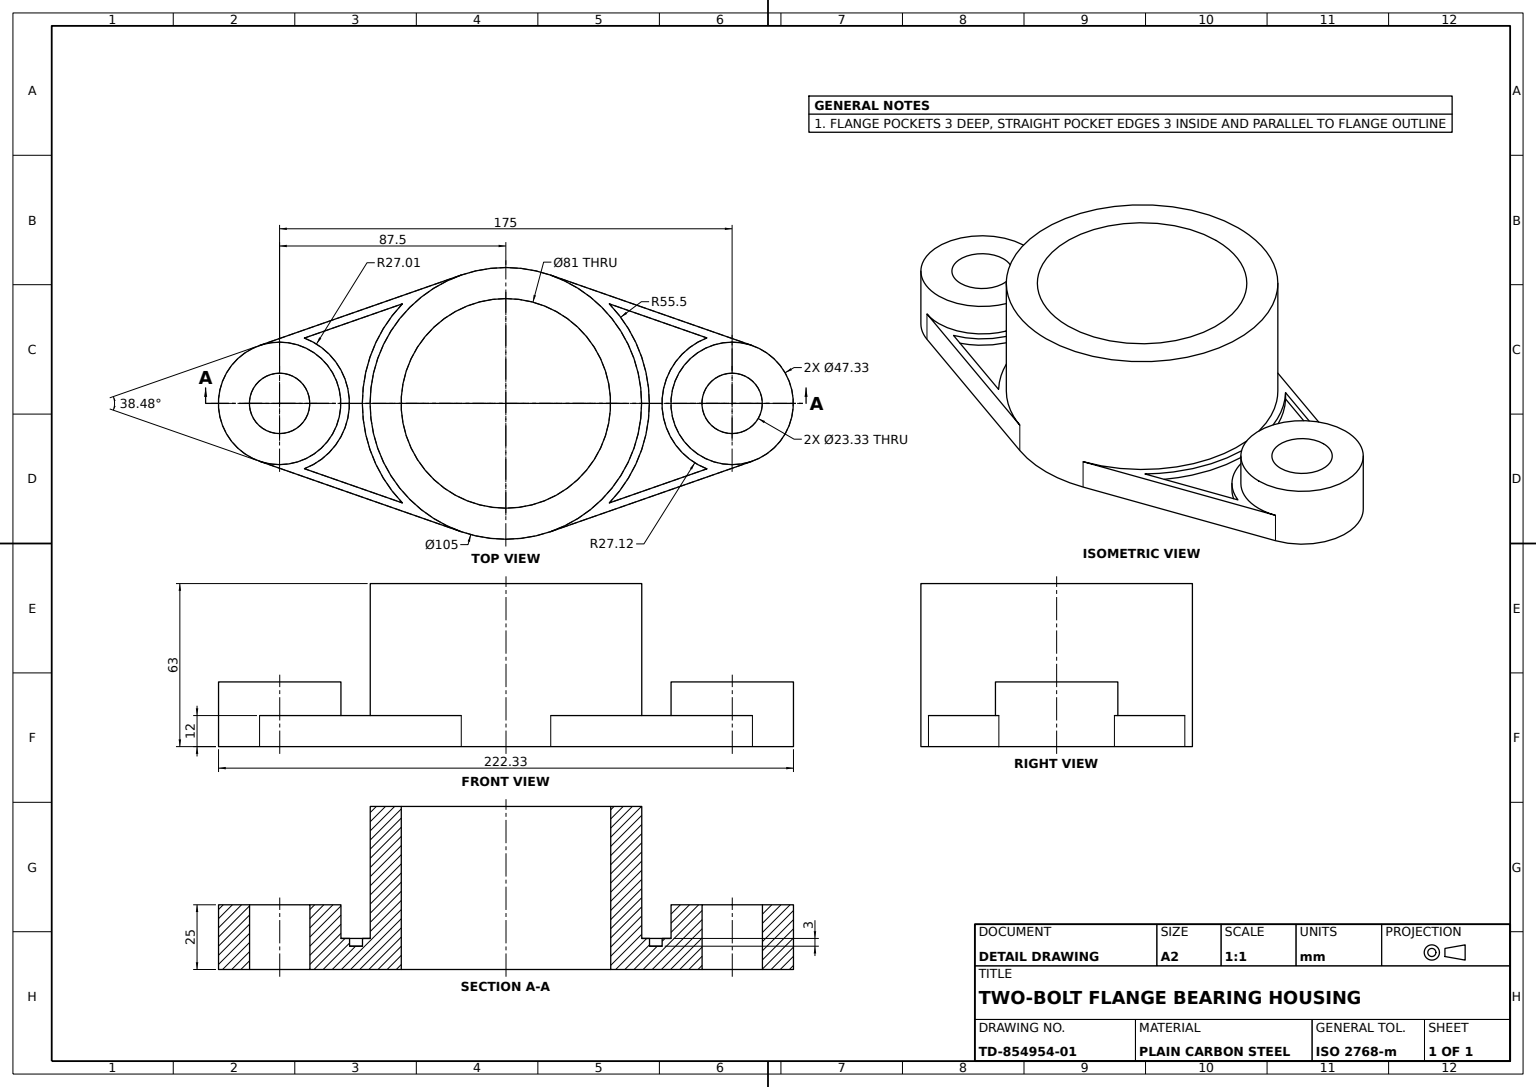
from build123d import *

# Parameters (mm, degrees)
HOUSING_PROFILE_SKETCH_R      = 52.5
HOUSING_PROFILE_SKETCH_R_2    = 40.5
BEARING_HOUSING_BOSS_DEPTH    = 63
MOUNTING_FLANGE_12MM_DEPTH    = 12
SKETCH1_4_R                   = 23.666666665
SKETCH1_4_R_2                 = 11.666666665
BOLT_LUG_BOSSES_25MM_DEPTH    = 25
FLANGE_POCKETS_3MM_DEEP_DEPTH = 3


with BuildPart() as part:
    # Housing Profile Sketch → Bearing Housing Boss (new body)
    with BuildSketch(Plane(origin=(0, 0, 0), x_dir=(1, 0, 0), z_dir=(0, 1, 0))):
        with Locations(Location((0, 0, 0), (0, 0, 270))):
            Circle(HOUSING_PROFILE_SKETCH_R)
        with Locations(Location((0, 0, 0), (0, 0, 270))):
            Circle(HOUSING_PROFILE_SKETCH_R_2, mode=Mode.SUBTRACT)
    extrude(amount=BEARING_HOUSING_BOSS_DEPTH)

    # Sketch1_3 → Mounting Flange 12mm (add)
    with BuildSketch(Plane(origin=(0, 0, 0), x_dir=(1, 0, 0), z_dir=(0, 1, 0))):
        with BuildLine():
            ThreePointArc((-17.300000001, -49.567731439), (-52.5, 0), (-17.300000001, 49.567731439))
            Line((-17.300000001, 49.567731439), (-95.298730159, 22.344818615))
            ThreePointArc((-95.298730159, 22.344818615), (-73.797059367, 19.296127307), (-63.833333335, 0))
            ThreePointArc((-63.833333335, 0), (-73.797059367, -19.296127307), (-95.298730159, -22.344818615))
            Line((-95.298730159, -22.344818615), (-17.300000001, -49.567731439))
        make_face()
        with BuildLine():
            Line((95.298730159, 22.344818615), (17.300000001, 49.567731439))
            ThreePointArc((17.300000001, 49.567731439), (42.804789452, 30.397368307), (52.5, 0))
            ThreePointArc((52.5, 0), (42.804789452, -30.397368307), (17.300000001, -49.567731439))
            Line((17.300000001, -49.567731439), (95.298730159, -22.344818615))
            ThreePointArc((95.298730159, -22.344818615), (63.833333335, 0), (95.298730159, 22.344818615))
        make_face()
    extrude(amount=MOUNTING_FLANGE_12MM_DEPTH)

    # Sketch1_4 → Bolt Lug Bosses 25mm (add)
    # profile 1 of 2: a face of its own
    with BuildSketch(Plane(origin=(0, 0, 0), x_dir=(1, 0, 0), z_dir=(0, 1, 0))):
        with Locations(Location((-87.5, 0, 0), (0, 0, 109.239875226))):
            Circle(SKETCH1_4_R)
        with Locations(Location((-87.5, 0, 0), (0, 0, 270))):
            Circle(SKETCH1_4_R_2, mode=Mode.SUBTRACT)
    # profile 2 of 2: a face of its own
    with BuildSketch(Plane(origin=(0, 0, 0), x_dir=(1, 0, 0), z_dir=(0, 1, 0))):
        with Locations(Location((87.5, 0, 0), (0, 0, 70.760124774))):
            Circle(SKETCH1_4_R)
        with Locations(Location((87.5, 0, 0), (0, 0, 270))):
            Circle(SKETCH1_4_R_2, mode=Mode.SUBTRACT)
    extrude(amount=BOLT_LUG_BOSSES_25MM_DEPTH)

    # Flange Pocket Sketch → Flange Pockets 3mm Deep (cut)
    with BuildSketch(Plane(origin=(0, 12, 0), x_dir=(1, 0, 0), z_dir=(0, 1, 0))):
        with BuildLine():
            Line((-40.009336858, 38.464307665), (-77.89822284, 25.240427764))
            ThreePointArc((-77.89822284, 25.240427764), (-60.494939024, 0), (-77.89822284, -25.240427764))
            Line((-77.89822284, -25.240427764), (-40.009336858, -38.464307665))
            ThreePointArc((-40.009336858, -38.464307665), (-55.5, 0), (-40.009336858, 38.464307665))
        make_face()
        with BuildLine():
            Line((40.009336858, 38.464307665), (77.732740957, 25.298183818))
            ThreePointArc((77.732740957, 25.298183818), (60.381787417, 0), (77.732740957, -25.298183818))
            Line((77.732740957, -25.298183818), (40.009336858, -38.464307665))
            ThreePointArc((40.009336858, -38.464307665), (55.5, 0), (40.009336858, 38.464307665))
        make_face()
    extrude(amount=-FLANGE_POCKETS_3MM_DEEP_DEPTH, mode=Mode.SUBTRACT)


solid = part.part
